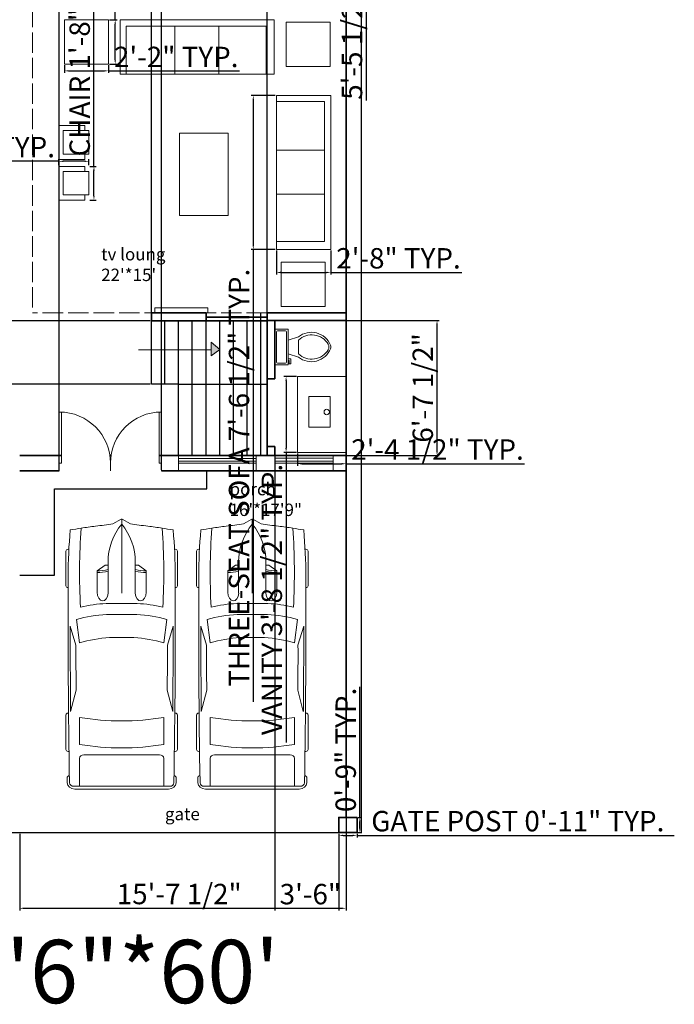
# Model space of a CAD drawing. Units: inches. Extents: x 3067 to 3879, y 3815 to 4813.
# Tile 2 of 3: x 3494 to 3879, y 3815 to 4395. Entities that reach past the tile are written whole.
import ezdxf

# ---------------------------------------------------------------- set-up
doc = ezdxf.new("R2010")
doc.units = ezdxf.units.IN
doc.linetypes.add('ACAD_ISO02W100', pattern=[15, 12, -3])
for name, color, linetype, lineweight in [('A-ANNO-DIMS', 2, 'Continuous', 18), ('A-ANNO-SYMB', 2, 'Continuous', 18), ('A-ANNO-TEXT', 7, 'Continuous', 25), ('A-AREA-IDEN', 7, 'Continuous', 18), ('A-COLS', 7, 'Continuous', 35), ('A-DOOR', 3, 'Continuous', 18), ('A-EQPM', 8, 'Continuous', 18), ('A-EQPM-VEHI', 9, 'Continuous', 13), ('A-FLOR-FIXT', 9, 'Continuous', 18), ('A-FLOR-OVHD', 8, 'ACAD_ISO02W100', 18), ('A-FLOR-STRS', 7, 'Continuous', 25), ('A-FURN', 8, 'Continuous', 18), ('A-GLAZ', 4, 'Continuous', 18), ('A-WALL', 7, 'Continuous', 35), ('C-PROP', 7, 'Continuous', 30)]:
    doc.layers.add(name, color=color, linetype=linetype, lineweight=lineweight)
doc.styles.get("Standard").update_dxf_attribs({"font": 'arial.ttf'})
doc.dimstyles.new('ISO-25', dxfattribs={"dimtxt": 12, "dimasz": 2.5, "dimexe": 1.25, "dimexo": 0.625, "dimtad": 1, "dimdec": 0, "dimlunit": 4, "dimtxsty": 'Standard', "dimcen": 2.5, "dimadec": 0, "dimazin": 0, "dimtfac": 1, "dimtdec": 0, "dimtmove": 0, "dimatfit": 3, "dimfxl": 1, "dimarcsym": 0})

# ---------------------------------------------------------------- blocks, each defined once
blk = doc.blocks.new('*U2')
for p, q in [((0, 0), (0, -6)), ((40, 0), (40, -6))]:
    blk.add_line(p, q)
blk.add_lwpolyline([(0, 0), (0, 40), (1.75, 40), (1.75, 0)], close=True)
blk.add_arc((0, 0), 40, 0, 90)
blk = doc.blocks.new('*U4')
for p, q in [((9.5, -6), (9.5, -2)), ((-10, -8.5), (-8, -8.5)), ((-10, -9.5), (-10, -8.5)), ((-7, -9.5), (-10, -9.5)), ((-8, -8.5), (-8, -8)), ((-7, -8), (-7, -9.5)), ((-4, -8), (-6, -14)), ((4, -8), (6, -14)), ((4, -14), (-4, -14))]:
    blk.add_line(p, q)
blk.add_lwpolyline([(10.5, -8), (10.5, 0), (-10.5, 0), (-10.5, -8)], close=True)
for points in [[(-9.5, -2), (-9.5, -6)], [(8.5, -1), (-8.5, -1)], [(-8.5, -7), (8.5, -7)]]:
    blk.add_lwpolyline(points)
for centre, radius, start, end in [((-8.62, -1.88), 0.884, 81.8699, 188.1301), ((8.62, -1.88), 0.884, 351.8699, 98.1301), ((-8.62, -6.12), 0.884, 171.8699, 278.1301), ((8.62, -6.12), 0.884, 261.8699, 8.1301), ((3.52, -21.58), 12.17, 141.46911, 247.97143), ((4.2, -21.82), 11.33, 136.36773, 238.94682), ((-3.52, -21.58), 12.17, 292.02843, 38.53071), ((-4.2, -21.82), 11.33, 301.05301, 43.63209), ((0, -27.88), 4, 245.73182, 294.26817), ((0, -29), 4, 254.86053, 285.13947)]:
    blk.add_arc(centre, radius, start, end)
blk = doc.blocks.new('*U6')
for p, q in [((21.1, 37.41), (21.1, 36.83)), ((46.55, 38.89), (22.35, 38.89)), ((47.8, 37.39), (47.8, 37.41)), ((87.99, 31.87), (74.76, 35.92)), ((134.31, 35.6), (119.29, 31.78)), ((135.45, 37.07), (135.45, 37.41)), ((136.7, 38.89), (160.9, 38.89)), ((162.15, 37.41), (162.15, 36.77)), ((70.03, 31.54), (86.41, 29.35)), ((138.42, 29.35), (157.25, 29.35)), ((186.47, 29.35), (167.01, 29.35)), ((186.47, -33.5), (186.47, 33.5)), ((188.4, -32.76), (188.4, 32.76)), ((164.52, 26.39), (164.52, -26.39)), ((32.27, 11.63), (36.13, 17.17)), ((36.13, 17.17), (50.94, 17.17)), ((29.77, 9.51), (51.68, 9.51)), ((32.12, 9.51), (32.12, 11.15)), ((58.92, -10.77), (58.92, 10.77)), ((66.55, -10.53), (66.55, 10.53)), ((82.74, 8.5), (82.74, -8.5)), ((186.47, -10.53), (186.47, 10.53)), ((3.27, 6.13), (0.1, 0.41)), ((0, 0), (51.68, 0)), ((0.1, -0.41), (3.27, -6.13)), ((29.77, -9.51), (51.68, -9.51)), ((32.12, -9.51), (32.12, -11.15)), ((32.27, -11.63), (36.13, -17.17)), ((36.13, -17.17), (50.94, -17.17)), ((86.41, -29.35), (70.03, -31.54)), ((87.99, -31.87), (74.76, -35.92)), ((134.31, -35.6), (119.29, -31.78)), ((157.25, -29.35), (138.42, -29.35)), ((167.01, -29.35), (186.47, -29.35)), ((21.1, -37.41), (21.1, -36.83)), ((46.55, -38.89), (22.35, -38.89)), ((47.8, -37.39), (47.8, -37.41)), ((135.45, -37.07), (135.45, -37.41)), ((136.7, -38.89), (160.9, -38.89)), ((162.15, -37.41), (162.15, -36.77))]:
    blk.add_line(p, q)
for centre, major_axis, ratio, start_param, end_param in [((266.03, -27.52), (0, 313.31), 0.842304, 1.367076, 1.39176), ((41.19, -490.86), (0, 528.23), 0.842304, 0.00281, 0.075598), ((22.35, 37.41), (0, -1.48), 0.842304, 3.141593, 4.712389), ((64.48, -10555.62), (0, 10593.03), 0.842304, -0.013397, 0.002797), ((46.55, 37.41), (0, 1.48), 0.842304, -1.570796, 0), ((64.48, -10555.62), (0, -10591.55), 0.842304, 3.133765, 3.140441), ((136.7, 37.41), (0, -1.48), 0.842304, 3.141593, 4.712389), ((160.9, 37.41), (0, 1.48), 0.842304, -1.570796, 0), ((180.63, 35.84), (0, 2.22), 0.842304, -0.013017, 1.249894), ((64.48, -10556.36), (0, 10595.31), 0.842304, -0.013397, -0.013017), ((183.98, 33.5), (0, -2.96), 0.842304, 1.570796, 3.128196), ((183.98, 32.76), (0, -5.25), 0.842304, 1.570796, 3.128196), ((259.18, -27.52), (0, -305.3), 0.842304, 4.528606, 4.561838), ((37.47, -593.96), (0, -623.33), 0.842304, 3.096046, 3.200911), ((134.4, 5.39), (0, -89.78), 0.842304, 4.449482, 4.652344), ((135.29, 5.39), (0, 81.77), 0.842304, 1.245306, 1.50788), ((149.6, 2.8), (0, -79.58), 0.842304, 4.372215, 4.640744), ((95.79, -3666.35), (0, -3698.24), 0.842304, 3.134049, 3.144098), ((17.08, 0), (0, 147.02), 0.842304, 4.511394, 4.913384), ((35.91, 0), (0, 147.02), 0.842304, 4.511394, 4.913384), ((167.01, 26.39), (0, 2.96), 0.842304, 0, 1.570796), ((-204.49, 52.4), (0, -250.96), 0.842304, 1.385369, 1.434372), ((13.04, 17.01), (0, 27.42), 0.842304, 4.435146, 4.718221), ((14.2, 17.01), (0, 27.42), 0.842304, 4.435146, 4.718221), ((50.79, 13.34), (6.34, -0.36), 0.603834, -1.395552, 1.581315), ((29.77, -46.66), (0, 56.17), 0.842304, 0, 0.590319), ((32.75, 11.15), (0, 0.74), 0.842304, 0.879714, 1.570796), ((0.62, 0), (0, -0.74), 0.842304, 4.131459, 5.293319), ((-204.49, -52.4), (0, 250.96), 0.842304, -1.434372, -1.385369), ((29.77, 46.66), (0, 56.17), 0.842304, 2.551274, 3.141593), ((32.75, -11.15), (0, -0.74), 0.842304, 4.712389, 5.403472), ((13.04, -17.01), (0, -27.42), 0.842304, 1.564964, 1.848039), ((14.2, -17.01), (0, -27.42), 0.842304, 1.564964, 1.848039), ((134.4, -5.39), (0, -89.78), 0.842304, -1.510751, -1.307889), ((135.29, -5.39), (0, -81.77), 0.842304, -1.50788, -1.245306), ((149.6, -2.8), (0, -79.58), 0.842304, -1.499151, -1.230623), ((259.18, 27.52), (0, 305.3), 0.842304, 1.721348, 1.754579), ((167.01, -26.39), (0, -2.96), 0.842304, 4.712389, 6.283185), ((266.03, 27.52), (0, 313.31), 0.842304, 1.749832, 1.774517), ((37.47, 593.96), (0, -623.33), 0.842304, -0.059319, 0.045547), ((95.79, 3666.35), (0, -3698.24), 0.842304, -0.002505, 0.007544), ((183.98, -33.5), (0, 2.96), 0.842304, 3.15499, 4.712389), ((183.98, -32.76), (0, -5.25), 0.842304, 0.013397, 1.570796), ((41.19, 490.86), (0, -528.23), 0.842304, -0.075598, -0.00281), ((22.35, -37.41), (0, 1.48), 0.842304, 1.570796, 3.141593), ((64.48, 10555.62), (0, 10593.03), 0.842304, 3.138796, 3.15499), ((46.55, -37.41), (0, -1.48), 0.842304, 0, 1.570796), ((64.48, 10555.62), (0, -10591.55), 0.842304, 0.001152, 0.007828), ((136.7, -37.41), (0, -1.48), 0.842304, -1.570796, 0), ((160.9, -37.41), (0, 1.48), 0.842304, 3.141593, 4.712389), ((180.63, -35.84), (0, -2.22), 0.842304, -1.249894, 0.013017), ((64.48, 10556.36), (0, 10595.31), 0.842304, 3.15461, 3.15499)]:
    blk.add_ellipse(centre, major_axis=major_axis, ratio=ratio, start_param=start_param, end_param=end_param)
at = {"extrusion": (0, 0, -1)}
blk.add_ellipse((50.79, -13.34), major_axis=(6.34, 0.36), ratio=0.603834, start_param=-1.395552, end_param=1.581315, dxfattribs=at)
blk = doc.blocks.new('CHAIR')
for p, q in [((0, 2.39), (0, 17.59)), ((0, 17.59), (19.86, 17.59)), ((19.86, 17.59), (19.86, 2.43)), ((3.13, 2.39), (0, 2.39)), ((19.86, 2.43), (16.92, 2.43))]:
    blk.add_line(p, q)
blk.add_lwpolyline([(3.13, 15.05), (16.92, 15.05), (16.92, 0), (3.13, 0)], close=True)
blk = doc.blocks.new('SOFA-3-SEAT')
for p, q in [((0, 0), (0, 32.05)), ((0, 32.05), (6.29, 32.05)), ((3.6, 32.05), (90.53, 32.05)), ((90.53, 32.05), (90.53, 0)), ((3.6, 28.29), (3.6, 0)), ((32.14, 28.29), (32.14, 0)), ((58.01, 28.29), (58.01, 0)), ((3.6, 0), (0, 0)), ((90.53, 0), (85.88, 0))]:
    blk.add_line(p, q)
blk.add_lwpolyline([(3.6, 28.29), (85.88, 28.29), (85.88, 0), (3.6, 0)])
blk = doc.blocks.new('LOUNGE-SIDE-TABLE')
blk.add_lwpolyline([(0, 26.11), (25.9, 26.11), (25.9, 0), (0, 0)], close=True)
blk = doc.blocks.new('VANITY-BASIN')
for points in [[(0, 28.58), (44.74, 28.58), (44.74, 0), (0, 0)], [(11.93, 6.65), (29.93, 6.65), (29.93, 19.14), (11.93, 19.14)]]:
    blk.add_lwpolyline(points, close=True)
blk.add_circle((20.98, 17.18), 1.58)
blk = doc.blocks.new('GATE-POST')
blk.add_line((10.76, 9), (10.76, 0))
blk.add_lwpolyline([(10.76, 9), (0, 9), (0, 0), (10.76, 0)], close=True)
blk = doc.blocks.new('*D21')
at = {"layer": 'A-ANNO-DIMS', "color": 0, "lineweight": -2, "transparency": 16777216}
for p, q in [((3538.08, 4308.43), (3538.08, 4442)), ((3535.73, 4308.43), (3539.33, 4308.43)), ((3538.08, 4291.07), (3538.08, 4305.93)), ((3535.73, 4288.57), (3539.33, 4288.57))]:
    blk.add_line(p, q, dxfattribs=at)
at = {"layer": 'A-ANNO-DIMS', "color": 0, "lineweight": 100, "transparency": 16777216}
for points in [[(3537.67, 4305.93), (3538.5, 4305.93), (3538.08, 4308.43)], [(3537.67, 4291.07), (3538.5, 4291.07), (3538.08, 4288.57)]]:
    blk.add_solid(points, dxfattribs=at)
at = {"layer": 'Defpoints', "color": 0, "lineweight": 100, "transparency": 16777216}
for p in [(3535.11, 4308.43), (3538.08, 4308.43), (3535.11, 4288.57)]:
    blk.add_point(p, dxfattribs=at)
at = {"layer": 'A-ANNO-DIMS', "color": 0, "transparency": 16777216, "insert": (3531.25, 4376.46), "char_height": 12, "attachment_point": 5, "rotation": 90}
blk.add_mtext('CHAIR 1\'-8" TYP.', dxfattribs=at)
blk = doc.blocks.new('*D22')
at = {"layer": 'A-ANNO-DIMS', "color": 0, "lineweight": -2, "transparency": 16777216}
for p, q in [((3517.51, 4309.05), (3517.51, 4312.65)), ((3535.11, 4309.05), (3535.11, 4312.65)), ((3517.51, 4311.4), (3413.79, 4311.4)), ((3532.61, 4311.4), (3520.01, 4311.4))]:
    blk.add_line(p, q, dxfattribs=at)
at = {"layer": 'A-ANNO-DIMS', "color": 0, "lineweight": 100, "transparency": 16777216}
for points in [[(3520.01, 4311.82), (3520.01, 4310.99), (3517.51, 4311.4)], [(3532.61, 4311.82), (3532.61, 4310.99), (3535.11, 4311.4)]]:
    blk.add_solid(points, dxfattribs=at)
at = {"layer": 'Defpoints', "color": 0, "lineweight": 100, "transparency": 16777216}
for p in [(3517.51, 4311.4), (3517.51, 4308.43), (3535.11, 4308.43)]:
    blk.add_point(p, dxfattribs=at)
at = {"layer": 'A-ANNO-DIMS', "color": 0, "transparency": 16777216, "insert": (3464.4, 4318.23), "char_height": 12, "attachment_point": 5}
blk.add_mtext('1\'-5 1/2" TYP.', dxfattribs=at)
blk = doc.blocks.new('*D29')
at = {"layer": 'A-ANNO-DIMS', "color": 0, "lineweight": -2, "transparency": 16777216}
for p, q in [((3550.59, 4394.65), (3550.59, 4573.04)), ((3547.3, 4394.65), (3551.84, 4394.65)), ((3550.59, 4371.05), (3550.59, 4392.15)), ((3547.3, 4368.55), (3551.84, 4368.55))]:
    blk.add_line(p, q, dxfattribs=at)
at = {"layer": 'A-ANNO-DIMS', "color": 0, "lineweight": 100, "transparency": 16777216}
for points in [[(3550.17, 4392.15), (3551.01, 4392.15), (3550.59, 4394.65)], [(3550.17, 4371.05), (3551.01, 4371.05), (3550.59, 4368.55)]]:
    blk.add_solid(points, dxfattribs=at)
at = {"layer": 'Defpoints', "color": 0, "lineweight": 100, "transparency": 16777216}
for p in [(3546.67, 4394.65), (3550.59, 4394.65), (3546.67, 4368.55)]:
    blk.add_point(p, dxfattribs=at)
at = {"layer": 'A-ANNO-DIMS', "color": 0, "transparency": 16777216, "insert": (3543.76, 4485.1), "char_height": 12, "attachment_point": 5, "rotation": 90}
blk.add_mtext('SIDE TABLE 2\'-2" TYP.', dxfattribs=at)
blk = doc.blocks.new('*D30')
at = {"layer": 'A-ANNO-DIMS', "color": 0, "lineweight": -2, "transparency": 16777216}
for p, q in [((3520.78, 4367.92), (3520.78, 4363.38)), ((3523.28, 4364.63), (3544.17, 4364.63)), ((3546.67, 4367.92), (3546.67, 4363.38)), ((3546.67, 4364.63), (3623.78, 4364.63))]:
    blk.add_line(p, q, dxfattribs=at)
at = {"layer": 'A-ANNO-DIMS', "color": 0, "lineweight": 100, "transparency": 16777216}
for points in [[(3523.28, 4365.05), (3523.28, 4364.21), (3520.78, 4364.63)], [(3544.17, 4365.05), (3544.17, 4364.21), (3546.67, 4364.63)]]:
    blk.add_solid(points, dxfattribs=at)
at = {"layer": 'Defpoints', "color": 0, "lineweight": 100, "transparency": 16777216}
for p in [(3520.78, 4368.55), (3546.67, 4368.55), (3546.67, 4364.63)]:
    blk.add_point(p, dxfattribs=at)
at = {"layer": 'A-ANNO-DIMS', "color": 0, "transparency": 16777216, "insert": (3586.48, 4371.28), "char_height": 12, "attachment_point": 5}
blk.add_mtext('2\'-2" TYP.', dxfattribs=at)
blk = doc.blocks.new('*D31')
at = {"layer": 'A-ANNO-DIMS', "color": 0, "lineweight": -2, "transparency": 16777216}
for p, q in [((3657.2, 4184.84), (3649.87, 4184.84)), ((3651.12, 4182.34), (3651.12, 4142.6)), ((3657.2, 4140.1), (3649.87, 4140.1)), ((3651.12, 4140.1), (3651.12, 3969.42))]:
    blk.add_line(p, q, dxfattribs=at)
at = {"layer": 'A-ANNO-DIMS', "color": 0, "lineweight": 100, "transparency": 16777216}
for points in [[(3650.7, 4182.34), (3651.53, 4182.34), (3651.12, 4184.84)], [(3650.7, 4142.6), (3651.53, 4142.6), (3651.12, 4140.1)]]:
    blk.add_solid(points, dxfattribs=at)
at = {"layer": 'Defpoints', "color": 0, "lineweight": 100, "transparency": 16777216}
for p in [(3657.83, 4184.84), (3651.12, 4140.1), (3657.83, 4140.1)]:
    blk.add_point(p, dxfattribs=at)
at = {"layer": 'A-ANNO-DIMS', "color": 0, "transparency": 16777216, "insert": (3644.28, 4053.51), "char_height": 12, "attachment_point": 5, "rotation": 90}
blk.add_mtext('VANITY 3\'-8 1/2" TYP.', dxfattribs=at)
blk = doc.blocks.new('*D32')
at = {"layer": 'A-ANNO-DIMS', "color": 0, "lineweight": -2, "transparency": 16777216}
for p, q in [((3657.83, 4139.48), (3657.83, 4132.14)), ((3686.41, 4139.48), (3686.41, 4132.14)), ((3660.33, 4133.39), (3683.91, 4133.39)), ((3686.41, 4133.39), (3791.47, 4133.39))]:
    blk.add_line(p, q, dxfattribs=at)
at = {"layer": 'A-ANNO-DIMS', "color": 0, "lineweight": 100, "transparency": 16777216}
for points in [[(3660.33, 4133.81), (3660.33, 4132.97), (3657.83, 4133.39)], [(3683.91, 4133.81), (3683.91, 4132.97), (3686.41, 4133.39)]]:
    blk.add_solid(points, dxfattribs=at)
at = {"layer": 'Defpoints', "color": 0, "lineweight": 100, "transparency": 16777216}
for p in [(3657.83, 4140.1), (3686.41, 4140.1), (3686.41, 4133.39)]:
    blk.add_point(p, dxfattribs=at)
at = {"layer": 'A-ANNO-DIMS', "color": 0, "transparency": 16777216, "insert": (3740.19, 4140.22), "char_height": 12, "attachment_point": 5}
blk.add_mtext('2\'-4 1/2" TYP.', dxfattribs=at)
blk = doc.blocks.new('*D33')
at = {"layer": 'A-ANNO-DIMS', "color": 0, "lineweight": -2, "transparency": 16777216}
for p, q in [((3644.77, 4350.11), (3630.56, 4350.11)), ((3631.81, 4347.61), (3631.81, 4262.08)), ((3644.77, 4259.58), (3630.56, 4259.58)), ((3631.81, 4259.58), (3631.81, 3993.28))]:
    blk.add_line(p, q, dxfattribs=at)
at = {"layer": 'A-ANNO-DIMS', "color": 0, "lineweight": 100, "transparency": 16777216}
for points in [[(3631.4, 4347.61), (3632.23, 4347.61), (3631.81, 4350.11)], [(3631.4, 4262.08), (3632.23, 4262.08), (3631.81, 4259.58)]]:
    blk.add_solid(points, dxfattribs=at)
at = {"layer": 'Defpoints', "color": 0, "lineweight": 100, "transparency": 16777216}
for p in [(3645.39, 4350.11), (3631.81, 4259.58), (3645.39, 4259.58)]:
    blk.add_point(p, dxfattribs=at)
at = {"layer": 'A-ANNO-DIMS', "color": 0, "transparency": 16777216, "insert": (3624.98, 4125.18), "char_height": 12, "attachment_point": 5, "rotation": 90}
blk.add_mtext('THREE-SEAT SOFA 7\'-6 1/2" TYP.', dxfattribs=at)
blk = doc.blocks.new('*D34')
at = {"layer": 'A-ANNO-DIMS', "color": 0, "lineweight": -2, "transparency": 16777216}
for p, q in [((3645.39, 4258.96), (3645.39, 4244.75)), ((3677.44, 4258.96), (3677.44, 4244.75)), ((3647.89, 4246), (3674.94, 4246)), ((3677.44, 4246), (3754.54, 4246))]:
    blk.add_line(p, q, dxfattribs=at)
at = {"layer": 'A-ANNO-DIMS', "color": 0, "lineweight": 100, "transparency": 16777216}
for points in [[(3647.89, 4246.42), (3647.89, 4245.59), (3645.39, 4246)], [(3674.94, 4246.42), (3674.94, 4245.59), (3677.44, 4246)]]:
    blk.add_solid(points, dxfattribs=at)
at = {"layer": 'Defpoints', "color": 0, "lineweight": 100, "transparency": 16777216}
for p in [(3645.39, 4259.58), (3677.44, 4259.58), (3677.44, 4246)]:
    blk.add_point(p, dxfattribs=at)
at = {"layer": 'A-ANNO-DIMS', "color": 0, "transparency": 16777216, "insert": (3717.24, 4252.76), "char_height": 12, "attachment_point": 5}
blk.add_mtext('2\'-8" TYP.', dxfattribs=at)
blk = doc.blocks.new('*D36')
at = {"layer": 'A-ANNO-DIMS', "color": 0, "lineweight": -2, "transparency": 16777216}
for p, q in [((3687.03, 4517.5), (3699.54, 4517.5)), ((3698.29, 4515), (3698.29, 4454.55)), ((3687.03, 4452.05), (3699.54, 4452.05)), ((3698.29, 4452.05), (3698.29, 4347.19))]:
    blk.add_line(p, q, dxfattribs=at)
at = {"layer": 'A-ANNO-DIMS', "color": 0, "lineweight": 100, "transparency": 16777216}
for points in [[(3697.88, 4515), (3698.71, 4515), (3698.29, 4517.5)], [(3697.88, 4454.55), (3698.71, 4454.55), (3698.29, 4452.05)]]:
    blk.add_solid(points, dxfattribs=at)
at = {"layer": 'Defpoints', "color": 0, "lineweight": 100, "transparency": 16777216}
for p in [(3686.41, 4517.5), (3686.41, 4452.05), (3698.29, 4452.05)]:
    blk.add_point(p, dxfattribs=at)
at = {"layer": 'A-ANNO-DIMS', "color": 0, "transparency": 16777216, "insert": (3691.46, 4398.37), "char_height": 12, "attachment_point": 5, "rotation": 90}
blk.add_mtext('5\'-5 1/2" TYP.', dxfattribs=at)
blk = doc.blocks.new('*D43')
at = {"layer": 'A-ANNO-DIMS', "color": 0, "lineweight": -2, "transparency": 16777216}
for p, q in [((3682.11, 3915.65), (3682.11, 3913.41)), ((3684.61, 3914.66), (3690.37, 3914.66)), ((3692.87, 3915.65), (3692.87, 3913.41)), ((3692.87, 3914.66), (3879.5, 3914.66))]:
    blk.add_line(p, q, dxfattribs=at)
at = {"layer": 'A-ANNO-DIMS', "color": 0, "lineweight": 100, "transparency": 16777216}
for points in [[(3684.61, 3915.07), (3684.61, 3914.24), (3682.11, 3914.66)], [(3690.37, 3915.07), (3690.37, 3914.24), (3692.87, 3914.66)]]:
    blk.add_solid(points, dxfattribs=at)
at = {"layer": 'Defpoints', "color": 0, "lineweight": 100, "transparency": 16777216}
for p in [(3682.11, 3916.27), (3692.87, 3916.27), (3692.87, 3914.66)]:
    blk.add_point(p, dxfattribs=at)
at = {"layer": 'A-ANNO-DIMS', "color": 0, "transparency": 16777216, "insert": (3787.43, 3921.49), "char_height": 12, "attachment_point": 5}
blk.add_mtext('GATE POST 0\'-11" TYP.', dxfattribs=at)
blk = doc.blocks.new('*D44')
at = {"layer": 'A-ANNO-DIMS', "color": 0, "lineweight": -2, "transparency": 16777216}
for p, q in [((3694.49, 3925.27), (3694.49, 4002.17)), ((3693.5, 3925.27), (3695.74, 3925.27)), ((3694.49, 3918.77), (3694.49, 3922.77)), ((3693.5, 3916.27), (3695.74, 3916.27))]:
    blk.add_line(p, q, dxfattribs=at)
at = {"layer": 'A-ANNO-DIMS', "color": 0, "lineweight": 100, "transparency": 16777216}
for points in [[(3694.07, 3922.77), (3694.9, 3922.77), (3694.49, 3925.27)], [(3694.07, 3918.77), (3694.9, 3918.77), (3694.49, 3916.27)]]:
    blk.add_solid(points, dxfattribs=at)
at = {"layer": 'Defpoints', "color": 0, "lineweight": 100, "transparency": 16777216}
for p in [(3692.87, 3925.27), (3694.49, 3925.27), (3692.87, 3916.27)]:
    blk.add_point(p, dxfattribs=at)
at = {"layer": 'A-ANNO-DIMS', "color": 0, "transparency": 16777216, "insert": (3687.74, 3964.97), "char_height": 12, "attachment_point": 5, "rotation": 90}
blk.add_mtext('0\'-9" TYP.', dxfattribs=at)
blk = doc.blocks.new('*D45')
at = {"layer": 'A-ANNO-DIMS', "color": 0, "lineweight": -2, "transparency": 16777216}
for p, q in [((3644.41, 4137.65), (3644.41, 3870.52)), ((3686.41, 4137.65), (3686.41, 3870.52)), ((3646.91, 3871.77), (3683.91, 3871.77))]:
    blk.add_line(p, q, dxfattribs=at)
at = {"layer": 'A-ANNO-DIMS', "color": 0, "lineweight": 100, "transparency": 16777216}
for points in [[(3646.91, 3872.19), (3646.91, 3871.36), (3644.41, 3871.77)], [(3683.91, 3872.19), (3683.91, 3871.36), (3686.41, 3871.77)]]:
    blk.add_solid(points, dxfattribs=at)
at = {"layer": 'Defpoints', "color": 0, "lineweight": 100, "transparency": 16777216}
for p in [(3644.41, 4138.27), (3686.41, 4138.27), (3686.41, 3871.77)]:
    blk.add_point(p, dxfattribs=at)
at = {"layer": 'A-ANNO-DIMS', "color": 0, "transparency": 16777216, "insert": (3665.41, 3878.53), "char_height": 12, "attachment_point": 5}
blk.add_mtext('3\'-6"', dxfattribs=at)
blk = doc.blocks.new('*D46')
at = {"layer": 'A-ANNO-DIMS', "color": 0, "lineweight": -2, "transparency": 16777216}
for p, q in [((3687.03, 4217.77), (3741.16, 4217.77)), ((3739.91, 4140.77), (3739.91, 4215.27)), ((3687.03, 4138.27), (3741.16, 4138.27))]:
    blk.add_line(p, q, dxfattribs=at)
at = {"layer": 'A-ANNO-DIMS', "color": 0, "lineweight": 100, "transparency": 16777216}
for points in [[(3739.49, 4215.27), (3740.32, 4215.27), (3739.91, 4217.77)], [(3739.49, 4140.77), (3740.32, 4140.77), (3739.91, 4138.27)]]:
    blk.add_solid(points, dxfattribs=at)
at = {"layer": 'Defpoints', "color": 0, "lineweight": 100, "transparency": 16777216}
for p in [(3686.41, 4217.77), (3739.91, 4217.77), (3686.41, 4138.27)]:
    blk.add_point(p, dxfattribs=at)
at = {"layer": 'A-ANNO-DIMS', "color": 0, "transparency": 16777216, "insert": (3733.08, 4178.02), "char_height": 12, "attachment_point": 5, "rotation": 90}
blk.add_mtext('6\'-7 1/2"', dxfattribs=at)
blk = doc.blocks.new('*D47')
at = {"layer": 'A-ANNO-DIMS', "color": 0, "lineweight": -2, "transparency": 16777216}
for p, q in [((3571.86, 4180.9), (3571.86, 4733.02)), ((3574.36, 4731.77), (3637.41, 4731.77)), ((3639.91, 4180.9), (3639.91, 4733.02))]:
    blk.add_line(p, q, dxfattribs=at)
at = {"layer": 'A-ANNO-DIMS', "color": 0, "lineweight": 100, "transparency": 16777216}
for points in [[(3574.36, 4732.19), (3574.36, 4731.36), (3571.86, 4731.77)], [(3637.41, 4732.19), (3637.41, 4731.36), (3639.91, 4731.77)]]:
    blk.add_solid(points, dxfattribs=at)
at = {"layer": 'Defpoints', "color": 0, "lineweight": 100, "transparency": 16777216}
for p in [(3639.91, 4731.77), (3571.86, 4180.27), (3639.91, 4180.27)]:
    blk.add_point(p, dxfattribs=at)
at = {"layer": 'A-ANNO-DIMS', "color": 0, "transparency": 16777216, "insert": (3605.89, 4738.52), "char_height": 12, "attachment_point": 5}
blk.add_mtext('5\'-8"', dxfattribs=at)
blk = doc.blocks.new('*D48')
at = {"layer": 'A-ANNO-DIMS', "color": 0, "lineweight": -2, "transparency": 16777216}
for p, q in [((3200.91, 4217.55), (3200.91, 4281.15)), ((3571.24, 4217.55), (3199.66, 4217.55)), ((3200.91, 4182.77), (3200.91, 4215.05)), ((3571.24, 4180.27), (3199.66, 4180.27))]:
    blk.add_line(p, q, dxfattribs=at)
at = {"layer": 'A-ANNO-DIMS', "color": 0, "lineweight": 100, "transparency": 16777216}
for points in [[(3200.49, 4215.05), (3201.32, 4215.05), (3200.91, 4217.55)], [(3200.49, 4182.77), (3201.32, 4182.77), (3200.91, 4180.27)]]:
    blk.add_solid(points, dxfattribs=at)
at = {"layer": 'Defpoints', "color": 0, "lineweight": 100, "transparency": 16777216}
for p in [(3200.91, 4217.55), (3571.86, 4217.55), (3571.86, 4180.27)]:
    blk.add_point(p, dxfattribs=at)
at = {"layer": 'A-ANNO-DIMS', "color": 0, "transparency": 16777216, "insert": (3194.07, 4250.6), "char_height": 12, "attachment_point": 5, "rotation": 90}
blk.add_mtext('3\'-1 1/2"', dxfattribs=at)
blk = doc.blocks.new('*D49')
at = {"layer": 'A-ANNO-DIMS', "color": 0, "lineweight": -2, "transparency": 16777216}
for p, q in [((3494.41, 3915.65), (3494.41, 3870.52)), ((3682.11, 3915.65), (3682.11, 3870.52)), ((3496.91, 3871.77), (3679.61, 3871.77))]:
    blk.add_line(p, q, dxfattribs=at)
at = {"layer": 'A-ANNO-DIMS', "color": 0, "lineweight": 100, "transparency": 16777216}
for points in [[(3496.91, 3872.19), (3496.91, 3871.36), (3494.41, 3871.77)], [(3679.61, 3872.19), (3679.61, 3871.36), (3682.11, 3871.77)]]:
    blk.add_solid(points, dxfattribs=at)
at = {"layer": 'Defpoints', "color": 0, "lineweight": 100, "transparency": 16777216}
for p in [(3494.41, 3916.27), (3682.11, 3916.27), (3682.11, 3871.77)]:
    blk.add_point(p, dxfattribs=at)
at = {"layer": 'A-ANNO-DIMS', "color": 0, "transparency": 16777216, "insert": (3588.26, 3878.6), "char_height": 12, "attachment_point": 5}
blk.add_mtext('15\'-7 1/2"', dxfattribs=at)
blk = doc.blocks.new('*D50')
at = {"layer": 'A-ANNO-DIMS', "color": 0, "lineweight": -2, "transparency": 16777216}
for p, q in [((3517.72, 4129.9), (3517.72, 4733.02)), ((3520.22, 4731.77), (3575.32, 4731.77)), ((3577.82, 4129.9), (3577.82, 4733.02))]:
    blk.add_line(p, q, dxfattribs=at)
at = {"layer": 'A-ANNO-DIMS', "color": 0, "lineweight": 100, "transparency": 16777216}
for points in [[(3520.22, 4732.19), (3520.22, 4731.36), (3517.72, 4731.77)], [(3575.32, 4732.19), (3575.32, 4731.36), (3577.82, 4731.77)]]:
    blk.add_solid(points, dxfattribs=at)
at = {"layer": 'Defpoints', "color": 0, "lineweight": 100, "transparency": 16777216}
for p in [(3577.82, 4731.77), (3517.72, 4129.27), (3577.82, 4129.27)]:
    blk.add_point(p, dxfattribs=at)
at = {"layer": 'A-ANNO-DIMS', "color": 0, "transparency": 16777216, "insert": (3547.77, 4738.52), "char_height": 12, "attachment_point": 5}
blk.add_mtext('5\'-0"', dxfattribs=at)

msp = doc.modelspace()

# ---------------------------------------------------------------- hatches: boundary and pattern name
at = {"layer": 'A-ANNO-SYMB'}
h = msp.add_hatch(color=256, dxfattribs=at)
h.dxf.hatch_style = 1
h.paths.add_polyline_path([(3607.08, 4204.94), (3607.08, 4197.69), (3607.08, 4196.97), (3612.08, 4200.69)])

# ---------------------------------------------------------------- linework, layer by layer
for p, q in [((3607.08, 4200.43), (3607.08, 4204.94)), ((3607.08, 4204.94), (3607.08, 4197.69)), ((3612.08, 4200.69), (3607.08, 4204.94)), ((3564.2, 4200.43), (3607.08, 4200.43)), ((3607.08, 4196.97), (3612.08, 4200.69)), ((3607.08, 4197.69), (3607.08, 4196.97))]:
    msp.add_line(p, q, dxfattribs=at)
at = {"layer": 'A-EQPM'}
msp.add_lwpolyline([(3573.92, 4222.27), (3605.06, 4222.27), (3605.06, 4225.07), (3573.92, 4225.07)], close=True, dxfattribs=at)
at = {"layer": 'A-FLOR-OVHD'}
for p in [(3501.91, 4402.27), (3639.91, 4222.27)]:
    msp.add_line(p, (3501.91, 4222.27), dxfattribs=at)
at = {"layer": 'A-FLOR-STRS'}
for p, q in [((3571.86, 4180.27), (3571.86, 4222.27)), ((3604.01, 4138.27), (3604.01, 4219.62)), ((3636.3, 4138.27), (3636.3, 4222.27)), ((3579.86, 4180.27), (3579.86, 4217.55)), ((3587.86, 4138.27), (3587.86, 4217.55)), ((3595.94, 4138.27), (3595.94, 4217.55)), ((3612.08, 4138.27), (3612.08, 4217.55)), ((3620.15, 4138.27), (3620.15, 4217.55)), ((3628.22, 4138.27), (3628.22, 4217.55)), ((3587.86, 4180.27), (3571.86, 4180.27)), ((3587.86, 4180.27), (3639.91, 4180.27)), ((3604.44, 4118.68), (3604.44, 4129.27)), ((3514.9, 4067.77), (3514.9, 4118.68)), ((3514.9, 4118.68), (3604.44, 4118.68)), ((3494.41, 4067.77), (3514.9, 4067.77))]:
    msp.add_line(p, q, dxfattribs=at)
at = {"layer": 'A-FURN'}
msp.add_lwpolyline([(3616.95, 4327.93), (3588.33, 4327.93), (3588.33, 4279.54), (3616.95, 4279.54)], close=True, dxfattribs=at)
at = {"layer": 'A-GLAZ'}
for p, q in [((3587.91, 4136.57), (3633.52, 4136.57)), ((3587.91, 4134.87), (3633.52, 4134.87)), ((3587.91, 4133.77), (3633.52, 4133.77)), ((3644.75, 4136.73), (3678.74, 4136.73)), ((3644.75, 4134.97), (3678.74, 4134.97)), ((3644.75, 4133.77), (3678.74, 4133.77))]:
    msp.add_line(p, q, dxfattribs=at)
for points in [[(3587.91, 4129.27), (3633.52, 4129.27), (3633.52, 4138.27), (3587.91, 4138.27)], [(3644.75, 4129.27), (3678.74, 4129.27), (3678.74, 4138.27), (3644.75, 4138.27)]]:
    msp.add_lwpolyline(points, close=True, dxfattribs=at)
at = {"layer": 'A-WALL'}
for p, q in [((3686.41, 4402.27), (3686.41, 4222.27)), ((3604.01, 4218.58), (3604.01, 4222.27)), ((3686.41, 4222.27), (3639.91, 4222.27)), ((3639.91, 4216.96), (3639.91, 4222.27)), ((3686.41, 4217.77), (3639.91, 4217.77)), ((3639.91, 4138.27), (3639.91, 4217.77)), ((3644.41, 4183.28), (3644.41, 4217.77)), ((3686.41, 4217.77), (3686.41, 4133.77)), ((3639.91, 4183.28), (3644.41, 4183.28)), ((3639.91, 4143.49), (3644.41, 4143.49)), ((3644.41, 4138.27), (3644.41, 4143.49)), ((3519.03, 4138.27), (3494.41, 4138.27)), ((3548.11, 4138.27), (3547.43, 4138.27)), ((3686.41, 4138.27), (3576.51, 4138.27)), ((3517.72, 4129.27), (3494.41, 4129.27)), ((3686.41, 4129.27), (3577.82, 4129.27)), ((3686.41, 4129.27), (3639.91, 4129.27))]:
    msp.add_line(p, q, dxfattribs=at)
for points in [[(3686.41, 3925.27), (3686.41, 4562.77)], [(3604.01, 4219.62), (3604.01, 4217.55), (3571.86, 4217.55), (3571.86, 4222.27), (3604.01, 4222.27)]]:
    msp.add_lwpolyline(points, dxfattribs=at)
msp.add_lwpolyline([(3604.01, 4217.55), (3639.91, 4217.55), (3639.91, 4219.62), (3604.01, 4219.62)], close=True, dxfattribs=at)
at = {"layer": 'C-PROP'}
msp.add_lwpolyline([(3245.41, 3916.27), (3695.41, 3916.27), (3695.41, 4636.27), (3245.41, 4636.27)], close=True, dxfattribs=at)

# ---------------------------------------------------------------- block references
at = {"layer": 'A-COLS'}
msp.add_blockref('GATE-POST', (3682.11, 3916.27), dxfattribs=at)
at = {"layer": 'A-DOOR', "yscale": 0.7513109794592311, "zscale": 0.7513109794592311}
for p, xscale in [((3517.72, 4133.78), 0.7513109794592311), ((3577.82, 4133.78), -0.7513109794592311)]:
    msp.add_blockref('*U2', p, dxfattribs=dict(at, xscale=xscale))
at = {"layer": 'A-EQPM-VEHI', "xscale": 0.8433419010415212, "yscale": 0.8433419010415212, "zscale": 0.8433419010415212, "rotation": 270}
for p in [(3554.4, 4100.83), (3631.24, 4100.83)]:
    msp.add_blockref('*U6', p, dxfattribs=at)
at = {"layer": 'A-FLOR-FIXT'}
for name, p, rotation in [('*U4', (3644.41, 4202.12), 90), ('VANITY-BASIN', (3657.83, 4184.84), 270.0000000000004)]:
    msp.add_blockref(name, p, dxfattribs=dict(at, rotation=rotation))
at = {"layer": 'A-FURN'}
for name, p in [('LOUNGE-SIDE-TABLE', (3520.78, 4368.55)), ('SOFA-3-SEAT', (3553.48, 4362.68)), ('LOUNGE-SIDE-TABLE', (3651.19, 4367.17)), ('LOUNGE-SIDE-TABLE', (3648.19, 4226.01))]:
    msp.add_blockref(name, p, dxfattribs=at)
for name, p, rotation in [('SOFA-3-SEAT', (3645.39, 4350.11), 270.0000000000031), ('CHAIR', (3535.11, 4312.52), 89.99999999999444), ('CHAIR', (3535.11, 4288.57), 89.99999999999692)]:
    msp.add_blockref(name, p, dxfattribs=dict(at, rotation=rotation))

# ---------------------------------------------------------------- texts
at = {"layer": 'A-ANNO-TEXT', "attachment_point": 1}
for s, width, gutter_width, insert, char_height in [('gate', 269.495, 36.54, (3579.87, 3930.9), 7.308), ('2bhk 37\'6"*60\'', 1373.908, 186.29, (3299.99, 3853.16), 37.2582)]:
    msp.add_mtext_dynamic_manual_height_columns(s, width=width, gutter_width=gutter_width, heights=[0], dxfattribs=dict(at, insert=insert, char_height=char_height))
at = {"layer": 'A-AREA-IDEN', "char_height": 7.308, "attachment_point": 1}
for s, insert in [("tv loung\\P22'*15'", (3542.34, 4260.4)), ('porch\\P16\'*17\'9"', (3617.89, 4122.13))]:
    msp.add_mtext_dynamic_manual_height_columns(s, width=269.495, gutter_width=36.54, heights=[0], dxfattribs=dict(at, insert=insert))

# ---------------------------------------------------------------- dimensions: what is measured, and where the dimension line sits
at = {"layer": 'A-ANNO-DIMS'}
for base, p1, p2, picture, middle in [((3577.82, 4731.77), (3517.72, 4129.27), (3577.82, 4129.27), '*D50', (3547.77, 4738.52)), ((3639.9073, 4731.7725), (3571.865, 4180.2725), (3639.9073, 4180.2725), '*D47', (3605.8862, 4738.5244)), ((3686.41, 3871.77), (3644.41, 4138.27), (3686.41, 4138.27), '*D45', (3665.41, 3878.53)), ((3682.11, 3871.77), (3494.41, 3916.27), (3682.11, 3916.27), '*D49', (3588.26, 3878.6))]:
    dim = msp.add_linear_dim(base=base, p1=p1, p2=p2, dimstyle='ISO-25', override={"dimdec": 1, "dimlfac": 1, "dimrnd": 0, "dimzin": 1, "dimdsep": 46, "dimlunit": 4, "dimfrac": 2}, dxfattribs=at)
    dim.commit()
    dim.dimension.update_dxf_attribs({"geometry": picture, "text_midpoint": middle})
for base, p1, p2, angle, text, picture, middle in [((3550.59, 4394.65), (3546.67, 4368.55), (3546.67, 4394.65), 90, 'SIDE TABLE <> TYP.', '*D29', (3543.76, 4485.1)), ((3698.2935, 4452.0456), (3686.4073, 4517.4994), (3686.4073, 4452.0456), 270, '<> TYP.', '*D36', (3691.4639, 4398.3667)), ((3538.08, 4308.43), (3535.11, 4288.57), (3535.11, 4308.43), 90, 'CHAIR <> TYP.', '*D21', (3531.25, 4376.46)), ((3631.81, 4259.58), (3645.39, 4350.11), (3645.39, 4259.58), 270, 'THREE-SEAT SOFA <> TYP.', '*D33', (3624.98, 4125.18)), ((3517.51, 4311.4), (3535.11, 4308.43), (3517.51, 4308.43), 180, '<> TYP.', '*D22', (3464.4, 4318.23)), ((3677.4378, 4246.0034), (3645.3925, 4259.5825), (3677.4378, 4259.5825), 0, '<> TYP.', '*D34', (3717.2381, 4252.7552)), ((3651.12, 4140.1), (3657.83, 4184.84), (3657.83, 4140.1), 270, 'VANITY <> TYP.', '*D31', (3644.28, 4053.51)), ((3694.49, 3925.27), (3692.87, 3916.27), (3692.87, 3925.27), 90, '<> TYP.', '*D44', (3687.74, 3964.97))]:
    dim = msp.add_linear_dim(base=base, p1=p1, p2=p2, angle=angle, text=text, dimstyle='ISO-25', override={"dimdec": 1, "dimlfac": 1, "dimrnd": 0, "dimzin": 1, "dimdsep": 46, "dimlunit": 4, "dimfrac": 2}, dxfattribs=at)
    dim.commit()
    dim.dimension.update_dxf_attribs({"geometry": picture, "text_midpoint": middle})
for base, p1, p2, text, picture, middle in [((3546.67, 4364.63), (3520.78, 4368.55), (3546.67, 4368.55), '<> TYP.', '*D30', (3586.48, 4371.28)), ((3686.41, 4133.39), (3657.83, 4140.1), (3686.41, 4140.1), '<> TYP.', '*D32', (3740.19, 4140.22)), ((3692.87, 3914.66), (3682.11, 3916.27), (3692.87, 3916.27), 'GATE POST <> TYP.', '*D43', (3787.43, 3921.49))]:
    dim = msp.add_linear_dim(base=base, p1=p1, p2=p2, text=text, dimstyle='ISO-25', override={"dimdec": 1, "dimlfac": 1, "dimrnd": 0, "dimzin": 1, "dimdsep": 46, "dimlunit": 4, "dimfrac": 2}, dxfattribs=at)
    dim.commit()
    dim.dimension.update_dxf_attribs({"geometry": picture, "text_midpoint": middle})
for base, p1, p2, picture, middle in [((3200.91, 4217.55), (3571.86, 4180.27), (3571.86, 4217.55), '*D48', (3194.07, 4250.6)), ((3739.91, 4217.77), (3686.41, 4138.27), (3686.41, 4217.77), '*D46', (3733.08, 4178.02))]:
    dim = msp.add_linear_dim(base=base, p1=p1, p2=p2, angle=90, dimstyle='ISO-25', override={"dimdec": 1, "dimlfac": 1, "dimrnd": 0, "dimzin": 1, "dimdsep": 46, "dimlunit": 4, "dimfrac": 2}, dxfattribs=at)
    dim.commit()
    dim.dimension.update_dxf_attribs({"geometry": picture, "text_midpoint": middle})

doc.saveas('drawing.dxf')
